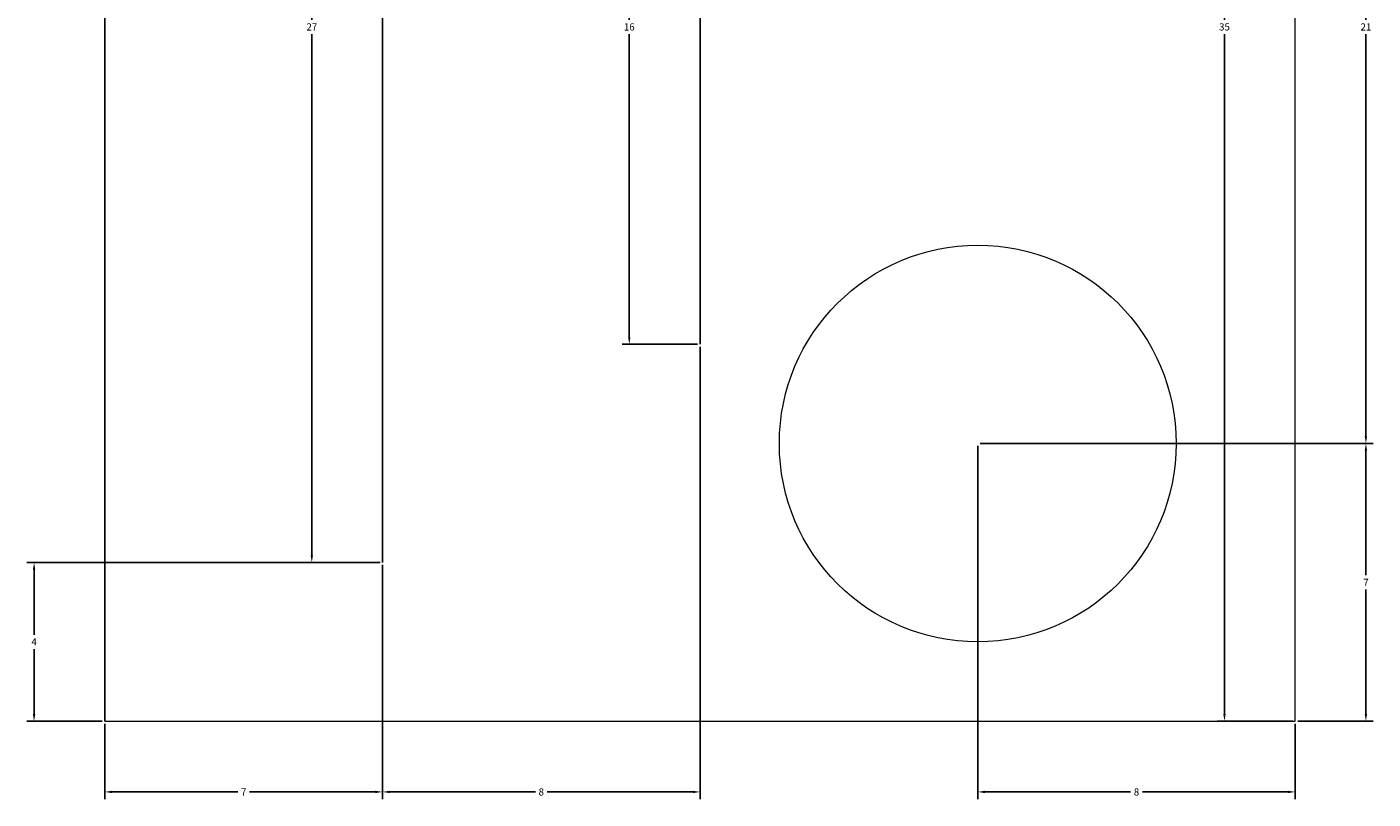
# Model space of a CAD drawing. Units: millimetres. Extents: x 136.9 to 170.9, y 96.9 to 135.8.
# Tile 1 of 2: x 136.9 to 170.9, y 96.9 to 116.3. Entities that reach past the tile are written whole.
import ezdxf

# ---------------------------------------------------------------- set-up
doc = ezdxf.new("R2010")
doc.units = ezdxf.units.MM
doc.layers.add('M-CONS', color=8, linetype='Continuous', lineweight=13)
doc.layers.add('M-DIMS', color=2, linetype='Continuous', lineweight=18)
doc.styles.get("Standard").update_dxf_attribs({"font": 'arial.ttf'})
doc.dimstyles.get("Standard").update_dxf_attribs({"dimtxt": 0.18, "dimasz": 0.18, "dimexe": 0.18, "dimexo": 0.0625, "dimgap": 0.09, "dimtad": 0, "dimtih": 1, "dimtoh": 1, "dimdec": 4, "dimzin": 0, "dimdsep": 46, "dimtxsty": 'Standard', "dimcen": 0.09, "dimadec": 0, "dimazin": 0, "dimtfac": 1, "dimtdec": 4, "dimtofl": 0, "dimtmove": 0, "dimatfit": 3, "dimfxl": 1, "dimtolj": 1, "dimtzin": 0, "dimarcsym": 0})

# ---------------------------------------------------------------- blocks, each defined once
blk = doc.blocks.new('*D2')
at = {"layer": 'Defpoints', "color": 0, "transparency": 16777216}
for p in [(167.107, 133.815), (168.89, 133.815), (168.89, 98.815)]:
    blk.add_point(p, dxfattribs=at)
at = {"layer": 'M-DIMS', "color": 0, "lineweight": -2, "transparency": 16777216}
for p, q in [((168.827, 133.815), (166.927, 133.815)), ((167.107, 133.635), (167.107, 116.497)), ((167.107, 98.995), (167.107, 116.133)), ((168.827, 98.815), (166.927, 98.815))]:
    blk.add_line(p, q, dxfattribs=at)
at = {"layer": 'M-DIMS', "color": 0, "transparency": 16777216}
for points in [[(167.077, 133.635), (167.137, 133.635), (167.107, 133.815)], [(167.077, 98.995), (167.137, 98.995), (167.107, 98.815)]]:
    blk.add_solid(points, dxfattribs=at)
at = {"layer": 'M-DIMS', "color": 0, "transparency": 16777216, "insert": (167.107, 116.315), "char_height": 0.18, "attachment_point": 5}
blk.add_mtext('\\A1;35', dxfattribs=at)
blk = doc.blocks.new('*D3')
at = {"layer": 'Defpoints', "color": 0, "transparency": 16777216}
for p in [(145.89, 102.816), (138.89, 98.815), (145.89, 97.033)]:
    blk.add_point(p, dxfattribs=at)
at = {"layer": 'M-DIMS', "color": 0, "lineweight": -2, "transparency": 16777216}
for p, q in [((145.89, 102.753), (145.89, 96.853)), ((138.89, 98.753), (138.89, 96.853)), ((139.07, 97.033), (142.241, 97.033)), ((145.71, 97.033), (142.538, 97.033))]:
    blk.add_line(p, q, dxfattribs=at)
at = {"layer": 'M-DIMS', "color": 0, "transparency": 16777216}
for points in [[(139.07, 97.063), (139.07, 97.003), (138.89, 97.033)], [(145.71, 97.063), (145.71, 97.003), (145.89, 97.033)]]:
    blk.add_solid(points, dxfattribs=at)
at = {"layer": 'M-DIMS', "color": 0, "transparency": 16777216, "insert": (142.39, 97.033), "char_height": 0.18, "attachment_point": 5}
blk.add_mtext('\\A1;7', dxfattribs=at)
blk = doc.blocks.new('*D4')
at = {"layer": 'Defpoints', "color": 0, "transparency": 16777216}
for p in [(153.89, 108.315), (145.89, 102.816), (153.89, 97.033)]:
    blk.add_point(p, dxfattribs=at)
at = {"layer": 'M-DIMS', "color": 0, "lineweight": -2, "transparency": 16777216}
for p, q in [((153.89, 108.253), (153.89, 96.853)), ((145.89, 102.753), (145.89, 96.853)), ((146.07, 97.033), (149.74, 97.033)), ((153.71, 97.033), (150.039, 97.033))]:
    blk.add_line(p, q, dxfattribs=at)
at = {"layer": 'M-DIMS', "color": 0, "transparency": 16777216}
for points in [[(146.07, 97.063), (146.07, 97.003), (145.89, 97.033)], [(153.71, 97.063), (153.71, 97.003), (153.89, 97.033)]]:
    blk.add_solid(points, dxfattribs=at)
at = {"layer": 'M-DIMS', "color": 0, "transparency": 16777216, "insert": (149.89, 97.033), "char_height": 0.18, "attachment_point": 5}
blk.add_mtext('\\A1;8', dxfattribs=at)
blk = doc.blocks.new('*D5')
at = {"layer": 'Defpoints', "color": 0, "transparency": 16777216}
for p in [(160.89, 105.815), (168.89, 98.815), (168.89, 97.033)]:
    blk.add_point(p, dxfattribs=at)
at = {"layer": 'M-DIMS', "color": 0, "lineweight": -2, "transparency": 16777216}
for p, q in [((160.89, 105.753), (160.89, 96.853)), ((168.89, 98.753), (168.89, 96.853)), ((161.07, 97.033), (164.74, 97.033)), ((168.71, 97.033), (165.039, 97.033))]:
    blk.add_line(p, q, dxfattribs=at)
at = {"layer": 'M-DIMS', "color": 0, "transparency": 16777216}
for points in [[(161.07, 97.063), (161.07, 97.003), (160.89, 97.033)], [(168.71, 97.063), (168.71, 97.003), (168.89, 97.033)]]:
    blk.add_solid(points, dxfattribs=at)
at = {"layer": 'M-DIMS', "color": 0, "transparency": 16777216, "insert": (164.89, 97.033), "char_height": 0.18, "attachment_point": 5}
blk.add_mtext('\\A1;8', dxfattribs=at)
blk = doc.blocks.new('*D6')
at = {"layer": 'Defpoints', "color": 0, "transparency": 16777216}
for p in [(137.107, 102.816), (145.89, 102.816), (138.89, 98.815)]:
    blk.add_point(p, dxfattribs=at)
at = {"layer": 'M-DIMS', "color": 0, "lineweight": -2, "transparency": 16777216}
for p, q in [((145.827, 102.816), (136.927, 102.816)), ((137.107, 102.636), (137.107, 100.995)), ((137.107, 98.995), (137.107, 100.635)), ((138.827, 98.815), (136.927, 98.815))]:
    blk.add_line(p, q, dxfattribs=at)
at = {"layer": 'M-DIMS', "color": 0, "transparency": 16777216}
for points in [[(137.077, 102.636), (137.137, 102.636), (137.107, 102.816)], [(137.077, 98.995), (137.137, 98.995), (137.107, 98.815)]]:
    blk.add_solid(points, dxfattribs=at)
at = {"layer": 'M-DIMS', "color": 0, "transparency": 16777216, "insert": (137.107, 100.815), "char_height": 0.18, "attachment_point": 5}
blk.add_mtext('\\A1;4', dxfattribs=at)
blk = doc.blocks.new('*D7')
at = {"layer": 'Defpoints', "color": 0, "transparency": 16777216}
for p in [(144.107, 129.815), (145.89, 129.815), (145.89, 102.816)]:
    blk.add_point(p, dxfattribs=at)
at = {"layer": 'M-DIMS', "color": 0, "lineweight": -2, "transparency": 16777216}
for p, q in [((145.827, 129.815), (143.927, 129.815)), ((144.107, 129.635), (144.107, 116.496)), ((144.107, 102.996), (144.107, 116.135)), ((145.827, 102.816), (143.927, 102.816))]:
    blk.add_line(p, q, dxfattribs=at)
at = {"layer": 'M-DIMS', "color": 0, "transparency": 16777216}
for points in [[(144.077, 129.635), (144.137, 129.635), (144.107, 129.815)], [(144.077, 102.996), (144.137, 102.996), (144.107, 102.816)]]:
    blk.add_solid(points, dxfattribs=at)
at = {"layer": 'M-DIMS', "color": 0, "transparency": 16777216, "insert": (144.107, 116.315), "char_height": 0.18, "attachment_point": 5}
blk.add_mtext('\\A1;27', dxfattribs=at)
blk = doc.blocks.new('*D8')
at = {"layer": 'Defpoints', "color": 0, "transparency": 16777216}
for p in [(152.107, 124.315), (153.89, 124.315), (153.89, 108.315)]:
    blk.add_point(p, dxfattribs=at)
at = {"layer": 'M-DIMS', "color": 0, "lineweight": -2, "transparency": 16777216}
for p, q in [((153.827, 124.315), (151.927, 124.315)), ((152.107, 124.135), (152.107, 116.497)), ((152.107, 108.495), (152.107, 116.133)), ((153.827, 108.315), (151.927, 108.315))]:
    blk.add_line(p, q, dxfattribs=at)
at = {"layer": 'M-DIMS', "color": 0, "transparency": 16777216}
for points in [[(152.077, 124.135), (152.137, 124.135), (152.107, 124.315)], [(152.077, 108.495), (152.137, 108.495), (152.107, 108.315)]]:
    blk.add_solid(points, dxfattribs=at)
at = {"layer": 'M-DIMS', "color": 0, "transparency": 16777216, "insert": (152.107, 116.315), "char_height": 0.18, "attachment_point": 5}
blk.add_mtext('\\A1;16', dxfattribs=at)
blk = doc.blocks.new('*D10')
at = {"layer": 'Defpoints', "color": 0, "transparency": 16777216}
for p in [(160.889688, 105.815309), (170.672188, 105.815309), (168.889688, 98.815309)]:
    blk.add_point(p, dxfattribs=at)
at = {"layer": 'M-DIMS', "color": 0, "lineweight": -2, "transparency": 16777216}
for p, q in [((160.952188, 105.815309), (170.852188, 105.815309)), ((170.672188, 105.635309), (170.672188, 102.495309)), ((170.672188, 98.995309), (170.672188, 102.135309)), ((168.952188, 98.815309), (170.852188, 98.815309))]:
    blk.add_line(p, q, dxfattribs=at)
at = {"layer": 'M-DIMS', "color": 0, "transparency": 16777216}
for points in [[(170.642188, 105.635309), (170.702188, 105.635309), (170.672188, 105.815309)], [(170.642188, 98.995309), (170.702188, 98.995309), (170.672188, 98.815309)]]:
    blk.add_solid(points, dxfattribs=at)
at = {"layer": 'M-DIMS', "color": 0, "transparency": 16777216, "insert": (170.672188, 102.315309), "char_height": 0.18, "attachment_point": 5}
blk.add_mtext('\\A1;7', dxfattribs=at)
blk = doc.blocks.new('*D11')
at = {"layer": 'Defpoints', "color": 0, "transparency": 16777216}
for p in [(160.89, 126.815), (170.672, 126.815), (160.89, 105.815)]:
    blk.add_point(p, dxfattribs=at)
at = {"layer": 'M-DIMS', "color": 0, "lineweight": -2, "transparency": 16777216}
for p, q in [((160.952, 126.815), (170.852, 126.815)), ((170.672, 126.635), (170.672, 116.496)), ((170.672, 105.995), (170.672, 116.135)), ((160.952, 105.815), (170.852, 105.815))]:
    blk.add_line(p, q, dxfattribs=at)
at = {"layer": 'M-DIMS', "color": 0, "transparency": 16777216}
for points in [[(170.642, 126.635), (170.702, 126.635), (170.672, 126.815)], [(170.642, 105.995), (170.702, 105.995), (170.672, 105.815)]]:
    blk.add_solid(points, dxfattribs=at)
at = {"layer": 'M-DIMS', "color": 0, "transparency": 16777216, "insert": (170.672, 116.315), "char_height": 0.18, "attachment_point": 5}
blk.add_mtext('\\A1;21', dxfattribs=at)

msp = doc.modelspace()

# ---------------------------------------------------------------- linework, layer by layer
at = {"layer": 'M-CONS'}
msp.add_lwpolyline([(168.89, 98.815), (168.89, 133.815), (138.89, 133.815), (138.89, 98.815)], close=True, dxfattribs=at)
at = {"layer": 'M-CONS', "extrusion": (1, -1e-16, 0), "elevation": 138.89}
msp.add_lwpolyline([(98.815, 55), (133.815, 55), (133.815, 0), (98.815, 0)], close=True, dxfattribs=at)
at = {"layer": 'M-CONS', "extrusion": (1, -1e-16, 0)}
msp.add_circle((116.315, 18.918, 153.89), 8, dxfattribs=at)
at = {"layer": 'M-CONS'}
msp.add_circle((160.89, 105.815), 5, dxfattribs=at)
at = {"layer": 'M-CONS', "extrusion": (1, 0, 1.7e-15)}
msp.add_rational_spline([(145.89, 113.315, 6.838), (145.89, 113.315, 3.419), (145.89, 113.315), (145.89, 114.815), (145.89, 116.315), (145.89, 117.815), (145.89, 119.315), (145.89, 119.315, 3.419), (145.89, 119.315, 6.838), (145.89, 131.08, 9.519), (145.89, 129.731, 21.509), (145.89, 128.382, 33.5), (145.89, 116.315, 33.5), (145.89, 104.249, 33.5), (145.89, 102.9, 21.509), (145.89, 101.551, 9.519), (145.89, 113.315, 6.838)], [1, 1, 1, 1, 1, 1, 1, 1, 1, 0.745591123387, 1, 0.745591123387, 1, 0.745591123387, 1, 0.745591123387, 1], degree=2, knots=[0, 0, 0, 1, 1, 2, 2, 3, 3, 4, 4, 5.45875, 5.45875, 6.9175, 6.9175, 8.376249, 8.376249, 9.834999, 9.834999, 9.834999], dxfattribs=at)

# ---------------------------------------------------------------- dimensions: what is measured, and where the dimension line sits
at = {"layer": 'M-DIMS'}
for base, p1, p2, picture, middle in [((167.107, 133.815), (168.89, 98.815), (168.89, 133.815), '*D2', (167.107, 116.315)), ((144.107, 129.815), (145.89, 102.816), (145.89, 129.815), '*D7', (144.107, 116.315)), ((170.672, 126.815), (160.89, 105.815), (160.89, 126.815), '*D11', (170.672, 116.315)), ((152.107, 124.315), (153.89, 108.315), (153.89, 124.315), '*D8', (152.107, 116.315)), ((170.672, 105.815), (168.89, 98.815), (160.89, 105.815), '*D10', (170.672, 102.315)), ((137.107, 102.816), (138.89, 98.815), (145.89, 102.816), '*D6', (137.107, 100.815))]:
    dim = msp.add_linear_dim(base=base, p1=p1, p2=p2, angle=90, dimstyle='Standard', override={"dimdec": 0, "dimlfac": 1, "dimrnd": 0, "dimzin": 0, "dimdsep": 46, "dimlunit": 2}, dxfattribs=at)
    dim.commit()
    dim.dimension.update_dxf_attribs({"geometry": picture, "text_midpoint": middle})
for base, p1, p2, picture, middle in [((153.89, 97.033), (145.89, 102.816), (153.89, 108.315), '*D4', (149.89, 97.033)), ((168.89, 97.033), (160.89, 105.815), (168.89, 98.815), '*D5', (164.89, 97.033)), ((145.89, 97.033), (138.89, 98.815), (145.89, 102.816), '*D3', (142.39, 97.033))]:
    dim = msp.add_linear_dim(base=base, p1=p1, p2=p2, dimstyle='Standard', override={"dimdec": 0, "dimlfac": 1, "dimrnd": 0, "dimzin": 0, "dimdsep": 46, "dimlunit": 2}, dxfattribs=at)
    dim.commit()
    dim.dimension.update_dxf_attribs({"geometry": picture, "text_midpoint": middle})

doc.saveas('drawing.dxf')
